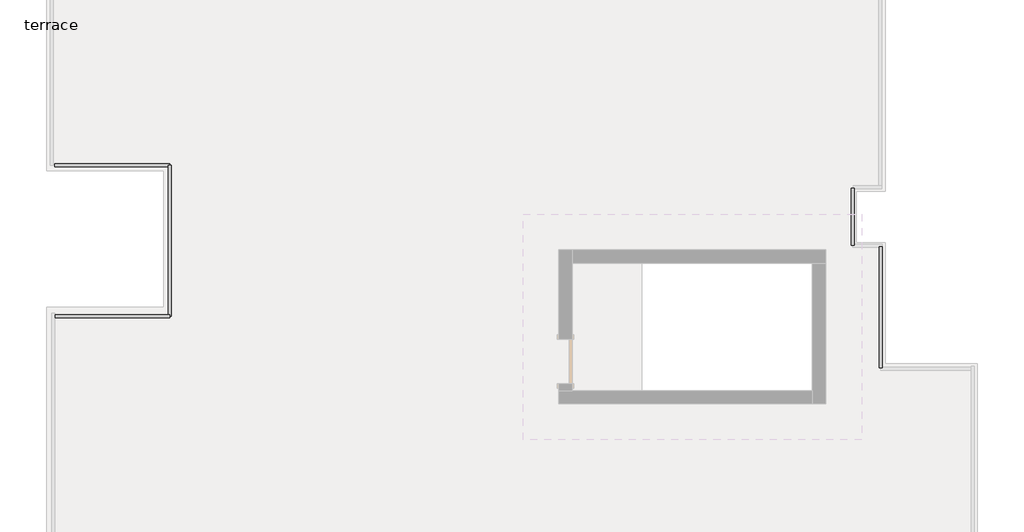
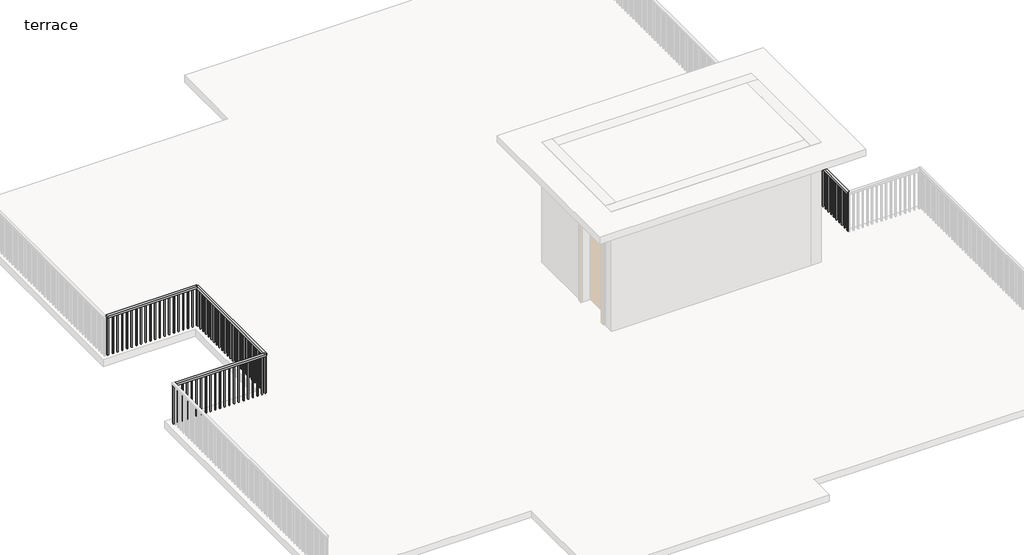
# One storey, part 4 of 7: 5 railings.
"""IFC4 building model written with IfcOpenShell, lengths in millimetres."""

from ifc_helpers import new_model, si_unit, frame, origin, place, context, project, spatial, polyline, outline, extrude, element, save

model = new_model("IFC4")

# Units and contexts
model_context = context("Model", 3, world=origin())
ifc_project = project(units=[si_unit("LENGTHUNIT", "METRE", prefix="MILLI")], contexts=[model_context])

# Site, building, storey
site = spatial("IfcSite", under=ifc_project)
building = spatial("IfcBuilding", under=site)
storey = spatial("IfcBuildingStorey", under=building, Name="terrace", Elevation=3810.0)

# Railings
placement = place(None, origin())
element("IfcRailing", 1, ObjectType="Handrail - Rectangular", at=placement, inside=storey, context=model_context, shape_type="SweptSolid", body=[
    extrude(outline(polyline([(-777.1890129, 5140.627622), (-726.3890129, 5140.627622), (-726.3890129, 4169.077622), (-777.1890129, 4169.077622), (-777.1890129, 5140.627622)])), frame((0.0, 0.0, 4673.6), z_axis=(0.0, 0.0, 1.0), x_axis=(1.0, 0.0, 0.0)), (0.0, 0.0, 1.0), 50.8),
    extrude(outline(polyline([(-761.3140129, 4235.752622), (-742.2640129, 4235.752622), (-742.2640129, 4216.702622), (-761.3140129, 4216.702622), (-761.3140129, 4235.752622)])), frame((0.0, 0.0, 3810.0), z_axis=(0.0, 0.0, 1.0), x_axis=(1.0, 0.0, 0.0)), (0.0, 0.0, 1.0), 863.6),
    extrude(outline(polyline([(-761.3140129, 4337.352622), (-742.2640129, 4337.352622), (-742.2640129, 4318.302622), (-761.3140129, 4318.302622), (-761.3140129, 4337.352622)])), frame((0.0, 0.0, 3810.0), z_axis=(0.0, 0.0, 1.0), x_axis=(1.0, 0.0, 0.0)), (0.0, 0.0, 1.0), 863.6),
    extrude(outline(polyline([(-761.3140129, 4438.952622), (-742.2640129, 4438.952622), (-742.2640129, 4419.902622), (-761.3140129, 4419.902622), (-761.3140129, 4438.952622)])), frame((0.0, 0.0, 3810.0), z_axis=(0.0, 0.0, 1.0), x_axis=(1.0, 0.0, 0.0)), (0.0, 0.0, 1.0), 863.6),
    extrude(outline(polyline([(-761.3140129, 4540.552622), (-742.2640129, 4540.552622), (-742.2640129, 4521.502622), (-761.3140129, 4521.502622), (-761.3140129, 4540.552622)])), frame((0.0, 0.0, 3810.0), z_axis=(0.0, 0.0, 1.0), x_axis=(1.0, 0.0, 0.0)), (0.0, 0.0, 1.0), 863.6),
    extrude(outline(polyline([(-761.3140129, 4642.152622), (-742.2640129, 4642.152622), (-742.2640129, 4623.102622), (-761.3140129, 4623.102622), (-761.3140129, 4642.152622)])), frame((0.0, 0.0, 3810.0), z_axis=(0.0, 0.0, 1.0), x_axis=(1.0, 0.0, 0.0)), (0.0, 0.0, 1.0), 863.6),
    extrude(outline(polyline([(-761.3140129, 4743.752622), (-742.2640129, 4743.752622), (-742.2640129, 4724.702622), (-761.3140129, 4724.702622), (-761.3140129, 4743.752622)])), frame((0.0, 0.0, 3810.0), z_axis=(0.0, 0.0, 1.0), x_axis=(1.0, 0.0, 0.0)), (0.0, 0.0, 1.0), 863.6),
    extrude(outline(polyline([(-761.3140129, 4845.352622), (-742.2640129, 4845.352622), (-742.2640129, 4826.302622), (-761.3140129, 4826.302622), (-761.3140129, 4845.352622)])), frame((0.0, 0.0, 3810.0), z_axis=(0.0, 0.0, 1.0), x_axis=(1.0, 0.0, 0.0)), (0.0, 0.0, 1.0), 863.6),
    extrude(outline(polyline([(-761.3140129, 4946.952622), (-742.2640129, 4946.952622), (-742.2640129, 4927.902622), (-761.3140129, 4927.902622), (-761.3140129, 4946.952622)])), frame((0.0, 0.0, 3810.0), z_axis=(0.0, 0.0, 1.0), x_axis=(1.0, 0.0, 0.0)), (0.0, 0.0, 1.0), 863.6),
    extrude(outline(polyline([(-761.3140129, 5048.552622), (-742.2640129, 5048.552622), (-742.2640129, 5029.502622), (-761.3140129, 5029.502622), (-761.3140129, 5048.552622)])), frame((0.0, 0.0, 3810.0), z_axis=(0.0, 0.0, 1.0), x_axis=(1.0, 0.0, 0.0)), (0.0, 0.0, 1.0), 863.6),
    extrude(outline(polyline([(-761.3140129, 4188.127622), (-742.2640129, 4188.127622), (-742.2640129, 4169.077622), (-761.3140129, 4169.077622), (-761.3140129, 4188.127622)])), frame((0.0, 0.0, 3810.0), z_axis=(0.0, 0.0, 1.0), x_axis=(1.0, 0.0, 0.0)), (0.0, 0.0, 1.0), 863.6),
    extrude(outline(polyline([(-761.3140129, 5140.627622), (-742.2640129, 5140.627622), (-742.2640129, 5121.577622), (-761.3140129, 5121.577622), (-761.3140129, 5140.627622)])), frame((0.0, 0.0, 3810.0), z_axis=(0.0, 0.0, 1.0), x_axis=(1.0, 0.0, 0.0)), (0.0, 0.0, 1.0), 863.6),
])
element("IfcRailing", 2, ObjectType="Handrail - Rectangular", at=placement, inside=storey, context=model_context, shape_type="SweptSolid", body=[
    extrude(outline(polyline([(-294.5890129, 4143.677622), (-243.7890129, 4143.677622), (-243.7890129, 2079.927622), (-294.5890129, 2079.927622), (-294.5890129, 4143.677622)])), frame((0.0, 0.0, 4673.6), z_axis=(0.0, 0.0, 1.0), x_axis=(1.0, 0.0, 0.0)), (0.0, 0.0, 1.0), 50.8),
    extrude(outline(polyline([(-278.7140129, 2121.202622), (-259.6640129, 2121.202622), (-259.6640129, 2102.152622), (-278.7140129, 2102.152622), (-278.7140129, 2121.202622)])), frame((0.0, 0.0, 3810.0), z_axis=(0.0, 0.0, 1.0), x_axis=(1.0, 0.0, 0.0)), (0.0, 0.0, 1.0), 863.6),
    extrude(outline(polyline([(-278.7140129, 2222.802622), (-259.6640129, 2222.802622), (-259.6640129, 2203.752622), (-278.7140129, 2203.752622), (-278.7140129, 2222.802622)])), frame((0.0, 0.0, 3810.0), z_axis=(0.0, 0.0, 1.0), x_axis=(1.0, 0.0, 0.0)), (0.0, 0.0, 1.0), 863.6),
    extrude(outline(polyline([(-278.7140129, 2324.402622), (-259.6640129, 2324.402622), (-259.6640129, 2305.352622), (-278.7140129, 2305.352622), (-278.7140129, 2324.402622)])), frame((0.0, 0.0, 3810.0), z_axis=(0.0, 0.0, 1.0), x_axis=(1.0, 0.0, 0.0)), (0.0, 0.0, 1.0), 863.6),
    extrude(outline(polyline([(-278.7140129, 2426.002622), (-259.6640129, 2426.002622), (-259.6640129, 2406.952622), (-278.7140129, 2406.952622), (-278.7140129, 2426.002622)])), frame((0.0, 0.0, 3810.0), z_axis=(0.0, 0.0, 1.0), x_axis=(1.0, 0.0, 0.0)), (0.0, 0.0, 1.0), 863.6),
    extrude(outline(polyline([(-278.7140129, 2527.602622), (-259.6640129, 2527.602622), (-259.6640129, 2508.552622), (-278.7140129, 2508.552622), (-278.7140129, 2527.602622)])), frame((0.0, 0.0, 3810.0), z_axis=(0.0, 0.0, 1.0), x_axis=(1.0, 0.0, 0.0)), (0.0, 0.0, 1.0), 863.6),
    extrude(outline(polyline([(-278.7140129, 2629.202622), (-259.6640129, 2629.202622), (-259.6640129, 2610.152622), (-278.7140129, 2610.152622), (-278.7140129, 2629.202622)])), frame((0.0, 0.0, 3810.0), z_axis=(0.0, 0.0, 1.0), x_axis=(1.0, 0.0, 0.0)), (0.0, 0.0, 1.0), 863.6),
    extrude(outline(polyline([(-278.7140129, 2730.802622), (-259.6640129, 2730.802622), (-259.6640129, 2711.752622), (-278.7140129, 2711.752622), (-278.7140129, 2730.802622)])), frame((0.0, 0.0, 3810.0), z_axis=(0.0, 0.0, 1.0), x_axis=(1.0, 0.0, 0.0)), (0.0, 0.0, 1.0), 863.6),
    extrude(outline(polyline([(-278.7140129, 2832.402622), (-259.6640129, 2832.402622), (-259.6640129, 2813.352622), (-278.7140129, 2813.352622), (-278.7140129, 2832.402622)])), frame((0.0, 0.0, 3810.0), z_axis=(0.0, 0.0, 1.0), x_axis=(1.0, 0.0, 0.0)), (0.0, 0.0, 1.0), 863.6),
    extrude(outline(polyline([(-278.7140129, 2934.002622), (-259.6640129, 2934.002622), (-259.6640129, 2914.952622), (-278.7140129, 2914.952622), (-278.7140129, 2934.002622)])), frame((0.0, 0.0, 3810.0), z_axis=(0.0, 0.0, 1.0), x_axis=(1.0, 0.0, 0.0)), (0.0, 0.0, 1.0), 863.6),
    extrude(outline(polyline([(-278.7140129, 3035.602622), (-259.6640129, 3035.602622), (-259.6640129, 3016.552622), (-278.7140129, 3016.552622), (-278.7140129, 3035.602622)])), frame((0.0, 0.0, 3810.0), z_axis=(0.0, 0.0, 1.0), x_axis=(1.0, 0.0, 0.0)), (0.0, 0.0, 1.0), 863.6),
    extrude(outline(polyline([(-278.7140129, 3137.202622), (-259.6640129, 3137.202622), (-259.6640129, 3118.152622), (-278.7140129, 3118.152622), (-278.7140129, 3137.202622)])), frame((0.0, 0.0, 3810.0), z_axis=(0.0, 0.0, 1.0), x_axis=(1.0, 0.0, 0.0)), (0.0, 0.0, 1.0), 863.6),
    extrude(outline(polyline([(-278.7140129, 3238.802622), (-259.6640129, 3238.802622), (-259.6640129, 3219.752622), (-278.7140129, 3219.752622), (-278.7140129, 3238.802622)])), frame((0.0, 0.0, 3810.0), z_axis=(0.0, 0.0, 1.0), x_axis=(1.0, 0.0, 0.0)), (0.0, 0.0, 1.0), 863.6),
    extrude(outline(polyline([(-278.7140129, 3340.402622), (-259.6640129, 3340.402622), (-259.6640129, 3321.352622), (-278.7140129, 3321.352622), (-278.7140129, 3340.402622)])), frame((0.0, 0.0, 3810.0), z_axis=(0.0, 0.0, 1.0), x_axis=(1.0, 0.0, 0.0)), (0.0, 0.0, 1.0), 863.6),
    extrude(outline(polyline([(-278.7140129, 3442.002622), (-259.6640129, 3442.002622), (-259.6640129, 3422.952622), (-278.7140129, 3422.952622), (-278.7140129, 3442.002622)])), frame((0.0, 0.0, 3810.0), z_axis=(0.0, 0.0, 1.0), x_axis=(1.0, 0.0, 0.0)), (0.0, 0.0, 1.0), 863.6),
    extrude(outline(polyline([(-278.7140129, 3543.602622), (-259.6640129, 3543.602622), (-259.6640129, 3524.552622), (-278.7140129, 3524.552622), (-278.7140129, 3543.602622)])), frame((0.0, 0.0, 3810.0), z_axis=(0.0, 0.0, 1.0), x_axis=(1.0, 0.0, 0.0)), (0.0, 0.0, 1.0), 863.6),
    extrude(outline(polyline([(-278.7140129, 3645.202622), (-259.6640129, 3645.202622), (-259.6640129, 3626.152622), (-278.7140129, 3626.152622), (-278.7140129, 3645.202622)])), frame((0.0, 0.0, 3810.0), z_axis=(0.0, 0.0, 1.0), x_axis=(1.0, 0.0, 0.0)), (0.0, 0.0, 1.0), 863.6),
    extrude(outline(polyline([(-278.7140129, 3746.802622), (-259.6640129, 3746.802622), (-259.6640129, 3727.752622), (-278.7140129, 3727.752622), (-278.7140129, 3746.802622)])), frame((0.0, 0.0, 3810.0), z_axis=(0.0, 0.0, 1.0), x_axis=(1.0, 0.0, 0.0)), (0.0, 0.0, 1.0), 863.6),
    extrude(outline(polyline([(-278.7140129, 3848.402622), (-259.6640129, 3848.402622), (-259.6640129, 3829.352622), (-278.7140129, 3829.352622), (-278.7140129, 3848.402622)])), frame((0.0, 0.0, 3810.0), z_axis=(0.0, 0.0, 1.0), x_axis=(1.0, 0.0, 0.0)), (0.0, 0.0, 1.0), 863.6),
    extrude(outline(polyline([(-278.7140129, 3950.002622), (-259.6640129, 3950.002622), (-259.6640129, 3930.952622), (-278.7140129, 3930.952622), (-278.7140129, 3950.002622)])), frame((0.0, 0.0, 3810.0), z_axis=(0.0, 0.0, 1.0), x_axis=(1.0, 0.0, 0.0)), (0.0, 0.0, 1.0), 863.6),
    extrude(outline(polyline([(-278.7140129, 4051.602622), (-259.6640129, 4051.602622), (-259.6640129, 4032.552622), (-278.7140129, 4032.552622), (-278.7140129, 4051.602622)])), frame((0.0, 0.0, 3810.0), z_axis=(0.0, 0.0, 1.0), x_axis=(1.0, 0.0, 0.0)), (0.0, 0.0, 1.0), 863.6),
    extrude(outline(polyline([(-278.7140129, 2098.977622), (-259.6640129, 2098.977622), (-259.6640129, 2079.927622), (-278.7140129, 2079.927622), (-278.7140129, 2098.977622)])), frame((0.0, 0.0, 3810.0), z_axis=(0.0, 0.0, 1.0), x_axis=(1.0, 0.0, 0.0)), (0.0, 0.0, 1.0), 863.6),
    extrude(outline(polyline([(-278.7140129, 4143.677622), (-259.6640129, 4143.677622), (-259.6640129, 4124.627622), (-278.7140129, 4124.627622), (-278.7140129, 4143.677622)])), frame((0.0, 0.0, 3810.0), z_axis=(0.0, 0.0, 1.0), x_axis=(1.0, 0.0, 0.0)), (0.0, 0.0, 1.0), 863.6),
])
element("IfcRailing", 3, ObjectType="Handrail - Rectangular", at=placement, inside=storey, context=model_context, shape_type="SweptSolid", body=[
    extrude(outline(polyline([(-14391.5890129, 2937.177622), (-14391.5890129, 2987.977622), (-12384.9890129, 2987.977622), (-12384.9890129, 2937.177622), (-14391.5890129, 2937.177622)])), frame((0.0, 0.0, 4673.6), z_axis=(0.0, 0.0, 1.0), x_axis=(1.0, 0.0, 0.0)), (0.0, 0.0, 1.0), 50.8),
    extrude(outline(polyline([(-12470.7140129, 2953.052622), (-12470.7140129, 2972.102622), (-12451.6640129, 2972.102622), (-12451.6640129, 2953.052622), (-12470.7140129, 2953.052622)])), frame((0.0, 0.0, 3810.0), z_axis=(0.0, 0.0, 1.0), x_axis=(1.0, 0.0, 0.0)), (0.0, 0.0, 1.0), 863.6),
    extrude(outline(polyline([(-12572.3140129, 2953.052622), (-12572.3140129, 2972.102622), (-12553.2640129, 2972.102622), (-12553.2640129, 2953.052622), (-12572.3140129, 2953.052622)])), frame((0.0, 0.0, 3810.0), z_axis=(0.0, 0.0, 1.0), x_axis=(1.0, 0.0, 0.0)), (0.0, 0.0, 1.0), 863.6),
    extrude(outline(polyline([(-12673.9140129, 2953.052622), (-12673.9140129, 2972.102622), (-12654.8640129, 2972.102622), (-12654.8640129, 2953.052622), (-12673.9140129, 2953.052622)])), frame((0.0, 0.0, 3810.0), z_axis=(0.0, 0.0, 1.0), x_axis=(1.0, 0.0, 0.0)), (0.0, 0.0, 1.0), 863.6),
    extrude(outline(polyline([(-12775.5140129, 2953.052622), (-12775.5140129, 2972.102622), (-12756.4640129, 2972.102622), (-12756.4640129, 2953.052622), (-12775.5140129, 2953.052622)])), frame((0.0, 0.0, 3810.0), z_axis=(0.0, 0.0, 1.0), x_axis=(1.0, 0.0, 0.0)), (0.0, 0.0, 1.0), 863.6),
    extrude(outline(polyline([(-12877.1140129, 2953.052622), (-12877.1140129, 2972.102622), (-12858.0640129, 2972.102622), (-12858.0640129, 2953.052622), (-12877.1140129, 2953.052622)])), frame((0.0, 0.0, 3810.0), z_axis=(0.0, 0.0, 1.0), x_axis=(1.0, 0.0, 0.0)), (0.0, 0.0, 1.0), 863.6),
    extrude(outline(polyline([(-12978.7140129, 2953.052622), (-12978.7140129, 2972.102622), (-12959.6640129, 2972.102622), (-12959.6640129, 2953.052622), (-12978.7140129, 2953.052622)])), frame((0.0, 0.0, 3810.0), z_axis=(0.0, 0.0, 1.0), x_axis=(1.0, 0.0, 0.0)), (0.0, 0.0, 1.0), 863.6),
    extrude(outline(polyline([(-13080.3140129, 2953.052622), (-13080.3140129, 2972.102622), (-13061.2640129, 2972.102622), (-13061.2640129, 2953.052622), (-13080.3140129, 2953.052622)])), frame((0.0, 0.0, 3810.0), z_axis=(0.0, 0.0, 1.0), x_axis=(1.0, 0.0, 0.0)), (0.0, 0.0, 1.0), 863.6),
    extrude(outline(polyline([(-13181.9140129, 2953.052622), (-13181.9140129, 2972.102622), (-13162.8640129, 2972.102622), (-13162.8640129, 2953.052622), (-13181.9140129, 2953.052622)])), frame((0.0, 0.0, 3810.0), z_axis=(0.0, 0.0, 1.0), x_axis=(1.0, 0.0, 0.0)), (0.0, 0.0, 1.0), 863.6),
    extrude(outline(polyline([(-13283.5140129, 2953.052622), (-13283.5140129, 2972.102622), (-13264.4640129, 2972.102622), (-13264.4640129, 2953.052622), (-13283.5140129, 2953.052622)])), frame((0.0, 0.0, 3810.0), z_axis=(0.0, 0.0, 1.0), x_axis=(1.0, 0.0, 0.0)), (0.0, 0.0, 1.0), 863.6),
    extrude(outline(polyline([(-13385.1140129, 2953.052622), (-13385.1140129, 2972.102622), (-13366.0640129, 2972.102622), (-13366.0640129, 2953.052622), (-13385.1140129, 2953.052622)])), frame((0.0, 0.0, 3810.0), z_axis=(0.0, 0.0, 1.0), x_axis=(1.0, 0.0, 0.0)), (0.0, 0.0, 1.0), 863.6),
    extrude(outline(polyline([(-13486.7140129, 2953.052622), (-13486.7140129, 2972.102622), (-13467.6640129, 2972.102622), (-13467.6640129, 2953.052622), (-13486.7140129, 2953.052622)])), frame((0.0, 0.0, 3810.0), z_axis=(0.0, 0.0, 1.0), x_axis=(1.0, 0.0, 0.0)), (0.0, 0.0, 1.0), 863.6),
    extrude(outline(polyline([(-13588.3140129, 2953.052622), (-13588.3140129, 2972.102622), (-13569.2640129, 2972.102622), (-13569.2640129, 2953.052622), (-13588.3140129, 2953.052622)])), frame((0.0, 0.0, 3810.0), z_axis=(0.0, 0.0, 1.0), x_axis=(1.0, 0.0, 0.0)), (0.0, 0.0, 1.0), 863.6),
    extrude(outline(polyline([(-13689.9140129, 2953.052622), (-13689.9140129, 2972.102622), (-13670.8640129, 2972.102622), (-13670.8640129, 2953.052622), (-13689.9140129, 2953.052622)])), frame((0.0, 0.0, 3810.0), z_axis=(0.0, 0.0, 1.0), x_axis=(1.0, 0.0, 0.0)), (0.0, 0.0, 1.0), 863.6),
    extrude(outline(polyline([(-13791.5140129, 2953.052622), (-13791.5140129, 2972.102622), (-13772.4640129, 2972.102622), (-13772.4640129, 2953.052622), (-13791.5140129, 2953.052622)])), frame((0.0, 0.0, 3810.0), z_axis=(0.0, 0.0, 1.0), x_axis=(1.0, 0.0, 0.0)), (0.0, 0.0, 1.0), 863.6),
    extrude(outline(polyline([(-13893.1140129, 2953.052622), (-13893.1140129, 2972.102622), (-13874.0640129, 2972.102622), (-13874.0640129, 2953.052622), (-13893.1140129, 2953.052622)])), frame((0.0, 0.0, 3810.0), z_axis=(0.0, 0.0, 1.0), x_axis=(1.0, 0.0, 0.0)), (0.0, 0.0, 1.0), 863.6),
    extrude(outline(polyline([(-13994.7140129, 2953.052622), (-13994.7140129, 2972.102622), (-13975.6640129, 2972.102622), (-13975.6640129, 2953.052622), (-13994.7140129, 2953.052622)])), frame((0.0, 0.0, 3810.0), z_axis=(0.0, 0.0, 1.0), x_axis=(1.0, 0.0, 0.0)), (0.0, 0.0, 1.0), 863.6),
    extrude(outline(polyline([(-14096.3140129, 2953.052622), (-14096.3140129, 2972.102622), (-14077.2640129, 2972.102622), (-14077.2640129, 2953.052622), (-14096.3140129, 2953.052622)])), frame((0.0, 0.0, 3810.0), z_axis=(0.0, 0.0, 1.0), x_axis=(1.0, 0.0, 0.0)), (0.0, 0.0, 1.0), 863.6),
    extrude(outline(polyline([(-14197.9140129, 2953.052622), (-14197.9140129, 2972.102622), (-14178.8640129, 2972.102622), (-14178.8640129, 2953.052622), (-14197.9140129, 2953.052622)])), frame((0.0, 0.0, 3810.0), z_axis=(0.0, 0.0, 1.0), x_axis=(1.0, 0.0, 0.0)), (0.0, 0.0, 1.0), 863.6),
    extrude(outline(polyline([(-14299.5140129, 2953.052622), (-14299.5140129, 2972.102622), (-14280.4640129, 2972.102622), (-14280.4640129, 2953.052622), (-14299.5140129, 2953.052622)])), frame((0.0, 0.0, 3810.0), z_axis=(0.0, 0.0, 1.0), x_axis=(1.0, 0.0, 0.0)), (0.0, 0.0, 1.0), 863.6),
    extrude(outline(polyline([(-12404.0390129, 2953.052622), (-12404.0390129, 2972.102622), (-12384.9890129, 2972.102622), (-12384.9890129, 2953.052622), (-12404.0390129, 2953.052622)])), frame((0.0, 0.0, 3810.0), z_axis=(0.0, 0.0, 1.0), x_axis=(1.0, 0.0, 0.0)), (0.0, 0.0, 1.0), 863.6),
    extrude(outline(polyline([(-14391.5890129, 2953.052622), (-14391.5890129, 2972.102622), (-14372.5390129, 2972.102622), (-14372.5390129, 2953.052622), (-14391.5890129, 2953.052622)])), frame((0.0, 0.0, 3810.0), z_axis=(0.0, 0.0, 1.0), x_axis=(1.0, 0.0, 0.0)), (0.0, 0.0, 1.0), 863.6),
])
element("IfcRailing", 4, ObjectType="Handrail - Rectangular", at=placement, inside=storey, context=model_context, shape_type="SweptSolid", body=[
    extrude(outline(polyline([(-12359.5890129, 2962.577622), (-12410.3890129, 2962.577622), (-12410.3890129, 5527.977622), (-12359.5890129, 5527.977622), (-12359.5890129, 2962.577622)])), frame((0.0, 0.0, 4673.6), z_axis=(0.0, 0.0, 1.0), x_axis=(1.0, 0.0, 0.0)), (0.0, 0.0, 1.0), 50.8),
    extrude(outline(polyline([(-12375.4640129, 5493.052622), (-12394.5140129, 5493.052622), (-12394.5140129, 5512.102622), (-12375.4640129, 5512.102622), (-12375.4640129, 5493.052622)])), frame((0.0, 0.0, 3810.0), z_axis=(0.0, 0.0, 1.0), x_axis=(1.0, 0.0, 0.0)), (0.0, 0.0, 1.0), 863.6),
    extrude(outline(polyline([(-12375.4640129, 5391.452622), (-12394.5140129, 5391.452622), (-12394.5140129, 5410.502622), (-12375.4640129, 5410.502622), (-12375.4640129, 5391.452622)])), frame((0.0, 0.0, 3810.0), z_axis=(0.0, 0.0, 1.0), x_axis=(1.0, 0.0, 0.0)), (0.0, 0.0, 1.0), 863.6),
    extrude(outline(polyline([(-12375.4640129, 5289.852622), (-12394.5140129, 5289.852622), (-12394.5140129, 5308.902622), (-12375.4640129, 5308.902622), (-12375.4640129, 5289.852622)])), frame((0.0, 0.0, 3810.0), z_axis=(0.0, 0.0, 1.0), x_axis=(1.0, 0.0, 0.0)), (0.0, 0.0, 1.0), 863.6),
    extrude(outline(polyline([(-12375.4640129, 5188.252622), (-12394.5140129, 5188.252622), (-12394.5140129, 5207.302622), (-12375.4640129, 5207.302622), (-12375.4640129, 5188.252622)])), frame((0.0, 0.0, 3810.0), z_axis=(0.0, 0.0, 1.0), x_axis=(1.0, 0.0, 0.0)), (0.0, 0.0, 1.0), 863.6),
    extrude(outline(polyline([(-12375.4640129, 5086.652622), (-12394.5140129, 5086.652622), (-12394.5140129, 5105.702622), (-12375.4640129, 5105.702622), (-12375.4640129, 5086.652622)])), frame((0.0, 0.0, 3810.0), z_axis=(0.0, 0.0, 1.0), x_axis=(1.0, 0.0, 0.0)), (0.0, 0.0, 1.0), 863.6),
    extrude(outline(polyline([(-12375.4640129, 4985.052622), (-12394.5140129, 4985.052622), (-12394.5140129, 5004.102622), (-12375.4640129, 5004.102622), (-12375.4640129, 4985.052622)])), frame((0.0, 0.0, 3810.0), z_axis=(0.0, 0.0, 1.0), x_axis=(1.0, 0.0, 0.0)), (0.0, 0.0, 1.0), 863.6),
    extrude(outline(polyline([(-12375.4640129, 4883.452622), (-12394.5140129, 4883.452622), (-12394.5140129, 4902.502622), (-12375.4640129, 4902.502622), (-12375.4640129, 4883.452622)])), frame((0.0, 0.0, 3810.0), z_axis=(0.0, 0.0, 1.0), x_axis=(1.0, 0.0, 0.0)), (0.0, 0.0, 1.0), 863.6),
    extrude(outline(polyline([(-12375.4640129, 4781.852622), (-12394.5140129, 4781.852622), (-12394.5140129, 4800.902622), (-12375.4640129, 4800.902622), (-12375.4640129, 4781.852622)])), frame((0.0, 0.0, 3810.0), z_axis=(0.0, 0.0, 1.0), x_axis=(1.0, 0.0, 0.0)), (0.0, 0.0, 1.0), 863.6),
    extrude(outline(polyline([(-12375.4640129, 4680.252622), (-12394.5140129, 4680.252622), (-12394.5140129, 4699.302622), (-12375.4640129, 4699.302622), (-12375.4640129, 4680.252622)])), frame((0.0, 0.0, 3810.0), z_axis=(0.0, 0.0, 1.0), x_axis=(1.0, 0.0, 0.0)), (0.0, 0.0, 1.0), 863.6),
    extrude(outline(polyline([(-12375.4640129, 4578.652622), (-12394.5140129, 4578.652622), (-12394.5140129, 4597.702622), (-12375.4640129, 4597.702622), (-12375.4640129, 4578.652622)])), frame((0.0, 0.0, 3810.0), z_axis=(0.0, 0.0, 1.0), x_axis=(1.0, 0.0, 0.0)), (0.0, 0.0, 1.0), 863.6),
    extrude(outline(polyline([(-12375.4640129, 4477.052622), (-12394.5140129, 4477.052622), (-12394.5140129, 4496.102622), (-12375.4640129, 4496.102622), (-12375.4640129, 4477.052622)])), frame((0.0, 0.0, 3810.0), z_axis=(0.0, 0.0, 1.0), x_axis=(1.0, 0.0, 0.0)), (0.0, 0.0, 1.0), 863.6),
    extrude(outline(polyline([(-12375.4640129, 4375.452622), (-12394.5140129, 4375.452622), (-12394.5140129, 4394.502622), (-12375.4640129, 4394.502622), (-12375.4640129, 4375.452622)])), frame((0.0, 0.0, 3810.0), z_axis=(0.0, 0.0, 1.0), x_axis=(1.0, 0.0, 0.0)), (0.0, 0.0, 1.0), 863.6),
    extrude(outline(polyline([(-12375.4640129, 4273.852622), (-12394.5140129, 4273.852622), (-12394.5140129, 4292.902622), (-12375.4640129, 4292.902622), (-12375.4640129, 4273.852622)])), frame((0.0, 0.0, 3810.0), z_axis=(0.0, 0.0, 1.0), x_axis=(1.0, 0.0, 0.0)), (0.0, 0.0, 1.0), 863.6),
    extrude(outline(polyline([(-12375.4640129, 4172.252622), (-12394.5140129, 4172.252622), (-12394.5140129, 4191.302622), (-12375.4640129, 4191.302622), (-12375.4640129, 4172.252622)])), frame((0.0, 0.0, 3810.0), z_axis=(0.0, 0.0, 1.0), x_axis=(1.0, 0.0, 0.0)), (0.0, 0.0, 1.0), 863.6),
    extrude(outline(polyline([(-12375.4640129, 4070.652622), (-12394.5140129, 4070.652622), (-12394.5140129, 4089.702622), (-12375.4640129, 4089.702622), (-12375.4640129, 4070.652622)])), frame((0.0, 0.0, 3810.0), z_axis=(0.0, 0.0, 1.0), x_axis=(1.0, 0.0, 0.0)), (0.0, 0.0, 1.0), 863.6),
    extrude(outline(polyline([(-12375.4640129, 3969.052622), (-12394.5140129, 3969.052622), (-12394.5140129, 3988.102622), (-12375.4640129, 3988.102622), (-12375.4640129, 3969.052622)])), frame((0.0, 0.0, 3810.0), z_axis=(0.0, 0.0, 1.0), x_axis=(1.0, 0.0, 0.0)), (0.0, 0.0, 1.0), 863.6),
    extrude(outline(polyline([(-12375.4640129, 3867.452622), (-12394.5140129, 3867.452622), (-12394.5140129, 3886.502622), (-12375.4640129, 3886.502622), (-12375.4640129, 3867.452622)])), frame((0.0, 0.0, 3810.0), z_axis=(0.0, 0.0, 1.0), x_axis=(1.0, 0.0, 0.0)), (0.0, 0.0, 1.0), 863.6),
    extrude(outline(polyline([(-12375.4640129, 3765.852622), (-12394.5140129, 3765.852622), (-12394.5140129, 3784.902622), (-12375.4640129, 3784.902622), (-12375.4640129, 3765.852622)])), frame((0.0, 0.0, 3810.0), z_axis=(0.0, 0.0, 1.0), x_axis=(1.0, 0.0, 0.0)), (0.0, 0.0, 1.0), 863.6),
    extrude(outline(polyline([(-12375.4640129, 3664.252622), (-12394.5140129, 3664.252622), (-12394.5140129, 3683.302622), (-12375.4640129, 3683.302622), (-12375.4640129, 3664.252622)])), frame((0.0, 0.0, 3810.0), z_axis=(0.0, 0.0, 1.0), x_axis=(1.0, 0.0, 0.0)), (0.0, 0.0, 1.0), 863.6),
    extrude(outline(polyline([(-12375.4640129, 3562.652622), (-12394.5140129, 3562.652622), (-12394.5140129, 3581.702622), (-12375.4640129, 3581.702622), (-12375.4640129, 3562.652622)])), frame((0.0, 0.0, 3810.0), z_axis=(0.0, 0.0, 1.0), x_axis=(1.0, 0.0, 0.0)), (0.0, 0.0, 1.0), 863.6),
    extrude(outline(polyline([(-12375.4640129, 3461.052622), (-12394.5140129, 3461.052622), (-12394.5140129, 3480.102622), (-12375.4640129, 3480.102622), (-12375.4640129, 3461.052622)])), frame((0.0, 0.0, 3810.0), z_axis=(0.0, 0.0, 1.0), x_axis=(1.0, 0.0, 0.0)), (0.0, 0.0, 1.0), 863.6),
    extrude(outline(polyline([(-12375.4640129, 3359.452622), (-12394.5140129, 3359.452622), (-12394.5140129, 3378.502622), (-12375.4640129, 3378.502622), (-12375.4640129, 3359.452622)])), frame((0.0, 0.0, 3810.0), z_axis=(0.0, 0.0, 1.0), x_axis=(1.0, 0.0, 0.0)), (0.0, 0.0, 1.0), 863.6),
    extrude(outline(polyline([(-12375.4640129, 3257.852622), (-12394.5140129, 3257.852622), (-12394.5140129, 3276.902622), (-12375.4640129, 3276.902622), (-12375.4640129, 3257.852622)])), frame((0.0, 0.0, 3810.0), z_axis=(0.0, 0.0, 1.0), x_axis=(1.0, 0.0, 0.0)), (0.0, 0.0, 1.0), 863.6),
    extrude(outline(polyline([(-12375.4640129, 3156.252622), (-12394.5140129, 3156.252622), (-12394.5140129, 3175.302622), (-12375.4640129, 3175.302622), (-12375.4640129, 3156.252622)])), frame((0.0, 0.0, 3810.0), z_axis=(0.0, 0.0, 1.0), x_axis=(1.0, 0.0, 0.0)), (0.0, 0.0, 1.0), 863.6),
    extrude(outline(polyline([(-12375.4640129, 3054.652622), (-12394.5140129, 3054.652622), (-12394.5140129, 3073.702622), (-12375.4640129, 3073.702622), (-12375.4640129, 3054.652622)])), frame((0.0, 0.0, 3810.0), z_axis=(0.0, 0.0, 1.0), x_axis=(1.0, 0.0, 0.0)), (0.0, 0.0, 1.0), 863.6),
    extrude(outline(polyline([(-12375.4640129, 5508.927622), (-12394.5140129, 5508.927622), (-12394.5140129, 5527.977622), (-12375.4640129, 5527.977622), (-12375.4640129, 5508.927622)])), frame((0.0, 0.0, 3810.0), z_axis=(0.0, 0.0, 1.0), x_axis=(1.0, 0.0, 0.0)), (0.0, 0.0, 1.0), 863.6),
    extrude(outline(polyline([(-12375.4640129, 2962.577622), (-12394.5140129, 2962.577622), (-12394.5140129, 2981.627622), (-12375.4640129, 2981.627622), (-12375.4640129, 2962.577622)])), frame((0.0, 0.0, 3810.0), z_axis=(0.0, 0.0, 1.0), x_axis=(1.0, 0.0, 0.0)), (0.0, 0.0, 1.0), 863.6),
])
element("IfcRailing", 5, ObjectType="Handrail - Rectangular", at=placement, inside=storey, context=model_context, shape_type="SweptSolid", body=[
    extrude(outline(polyline([(-12384.9890129, 5553.377622), (-12384.9890129, 5502.577622), (-14340.7890129, 5502.577622), (-14340.7890129, 5553.377622), (-12384.9890129, 5553.377622)])), frame((0.0, 0.0, 4673.6), z_axis=(0.0, 0.0, 1.0), x_axis=(1.0, 0.0, 0.0)), (0.0, 0.0, 1.0), 50.8),
    extrude(outline(polyline([(-14305.8640129, 5537.502622), (-14305.8640129, 5518.452622), (-14324.9140129, 5518.452622), (-14324.9140129, 5537.502622), (-14305.8640129, 5537.502622)])), frame((0.0, 0.0, 3810.0), z_axis=(0.0, 0.0, 1.0), x_axis=(1.0, 0.0, 0.0)), (0.0, 0.0, 1.0), 863.6),
    extrude(outline(polyline([(-14204.2640129, 5537.502622), (-14204.2640129, 5518.452622), (-14223.3140129, 5518.452622), (-14223.3140129, 5537.502622), (-14204.2640129, 5537.502622)])), frame((0.0, 0.0, 3810.0), z_axis=(0.0, 0.0, 1.0), x_axis=(1.0, 0.0, 0.0)), (0.0, 0.0, 1.0), 863.6),
    extrude(outline(polyline([(-14102.6640129, 5537.502622), (-14102.6640129, 5518.452622), (-14121.7140129, 5518.452622), (-14121.7140129, 5537.502622), (-14102.6640129, 5537.502622)])), frame((0.0, 0.0, 3810.0), z_axis=(0.0, 0.0, 1.0), x_axis=(1.0, 0.0, 0.0)), (0.0, 0.0, 1.0), 863.6),
    extrude(outline(polyline([(-14001.0640129, 5537.502622), (-14001.0640129, 5518.452622), (-14020.1140129, 5518.452622), (-14020.1140129, 5537.502622), (-14001.0640129, 5537.502622)])), frame((0.0, 0.0, 3810.0), z_axis=(0.0, 0.0, 1.0), x_axis=(1.0, 0.0, 0.0)), (0.0, 0.0, 1.0), 863.6),
    extrude(outline(polyline([(-13899.4640129, 5537.502622), (-13899.4640129, 5518.452622), (-13918.5140129, 5518.452622), (-13918.5140129, 5537.502622), (-13899.4640129, 5537.502622)])), frame((0.0, 0.0, 3810.0), z_axis=(0.0, 0.0, 1.0), x_axis=(1.0, 0.0, 0.0)), (0.0, 0.0, 1.0), 863.6),
    extrude(outline(polyline([(-13797.8640129, 5537.502622), (-13797.8640129, 5518.452622), (-13816.9140129, 5518.452622), (-13816.9140129, 5537.502622), (-13797.8640129, 5537.502622)])), frame((0.0, 0.0, 3810.0), z_axis=(0.0, 0.0, 1.0), x_axis=(1.0, 0.0, 0.0)), (0.0, 0.0, 1.0), 863.6),
    extrude(outline(polyline([(-13696.2640129, 5537.502622), (-13696.2640129, 5518.452622), (-13715.3140129, 5518.452622), (-13715.3140129, 5537.502622), (-13696.2640129, 5537.502622)])), frame((0.0, 0.0, 3810.0), z_axis=(0.0, 0.0, 1.0), x_axis=(1.0, 0.0, 0.0)), (0.0, 0.0, 1.0), 863.6),
    extrude(outline(polyline([(-13594.6640129, 5537.502622), (-13594.6640129, 5518.452622), (-13613.7140129, 5518.452622), (-13613.7140129, 5537.502622), (-13594.6640129, 5537.502622)])), frame((0.0, 0.0, 3810.0), z_axis=(0.0, 0.0, 1.0), x_axis=(1.0, 0.0, 0.0)), (0.0, 0.0, 1.0), 863.6),
    extrude(outline(polyline([(-13493.0640129, 5537.502622), (-13493.0640129, 5518.452622), (-13512.1140129, 5518.452622), (-13512.1140129, 5537.502622), (-13493.0640129, 5537.502622)])), frame((0.0, 0.0, 3810.0), z_axis=(0.0, 0.0, 1.0), x_axis=(1.0, 0.0, 0.0)), (0.0, 0.0, 1.0), 863.6),
    extrude(outline(polyline([(-13391.4640129, 5537.502622), (-13391.4640129, 5518.452622), (-13410.5140129, 5518.452622), (-13410.5140129, 5537.502622), (-13391.4640129, 5537.502622)])), frame((0.0, 0.0, 3810.0), z_axis=(0.0, 0.0, 1.0), x_axis=(1.0, 0.0, 0.0)), (0.0, 0.0, 1.0), 863.6),
    extrude(outline(polyline([(-13289.8640129, 5537.502622), (-13289.8640129, 5518.452622), (-13308.9140129, 5518.452622), (-13308.9140129, 5537.502622), (-13289.8640129, 5537.502622)])), frame((0.0, 0.0, 3810.0), z_axis=(0.0, 0.0, 1.0), x_axis=(1.0, 0.0, 0.0)), (0.0, 0.0, 1.0), 863.6),
    extrude(outline(polyline([(-13188.2640129, 5537.502622), (-13188.2640129, 5518.452622), (-13207.3140129, 5518.452622), (-13207.3140129, 5537.502622), (-13188.2640129, 5537.502622)])), frame((0.0, 0.0, 3810.0), z_axis=(0.0, 0.0, 1.0), x_axis=(1.0, 0.0, 0.0)), (0.0, 0.0, 1.0), 863.6),
    extrude(outline(polyline([(-13086.6640129, 5537.502622), (-13086.6640129, 5518.452622), (-13105.7140129, 5518.452622), (-13105.7140129, 5537.502622), (-13086.6640129, 5537.502622)])), frame((0.0, 0.0, 3810.0), z_axis=(0.0, 0.0, 1.0), x_axis=(1.0, 0.0, 0.0)), (0.0, 0.0, 1.0), 863.6),
    extrude(outline(polyline([(-12985.0640129, 5537.502622), (-12985.0640129, 5518.452622), (-13004.1140129, 5518.452622), (-13004.1140129, 5537.502622), (-12985.0640129, 5537.502622)])), frame((0.0, 0.0, 3810.0), z_axis=(0.0, 0.0, 1.0), x_axis=(1.0, 0.0, 0.0)), (0.0, 0.0, 1.0), 863.6),
    extrude(outline(polyline([(-12883.4640129, 5537.502622), (-12883.4640129, 5518.452622), (-12902.5140129, 5518.452622), (-12902.5140129, 5537.502622), (-12883.4640129, 5537.502622)])), frame((0.0, 0.0, 3810.0), z_axis=(0.0, 0.0, 1.0), x_axis=(1.0, 0.0, 0.0)), (0.0, 0.0, 1.0), 863.6),
    extrude(outline(polyline([(-12781.8640129, 5537.502622), (-12781.8640129, 5518.452622), (-12800.9140129, 5518.452622), (-12800.9140129, 5537.502622), (-12781.8640129, 5537.502622)])), frame((0.0, 0.0, 3810.0), z_axis=(0.0, 0.0, 1.0), x_axis=(1.0, 0.0, 0.0)), (0.0, 0.0, 1.0), 863.6),
    extrude(outline(polyline([(-12680.2640129, 5537.502622), (-12680.2640129, 5518.452622), (-12699.3140129, 5518.452622), (-12699.3140129, 5537.502622), (-12680.2640129, 5537.502622)])), frame((0.0, 0.0, 3810.0), z_axis=(0.0, 0.0, 1.0), x_axis=(1.0, 0.0, 0.0)), (0.0, 0.0, 1.0), 863.6),
    extrude(outline(polyline([(-12578.6640129, 5537.502622), (-12578.6640129, 5518.452622), (-12597.7140129, 5518.452622), (-12597.7140129, 5537.502622), (-12578.6640129, 5537.502622)])), frame((0.0, 0.0, 3810.0), z_axis=(0.0, 0.0, 1.0), x_axis=(1.0, 0.0, 0.0)), (0.0, 0.0, 1.0), 863.6),
    extrude(outline(polyline([(-12477.0640129, 5537.502622), (-12477.0640129, 5518.452622), (-12496.1140129, 5518.452622), (-12496.1140129, 5537.502622), (-12477.0640129, 5537.502622)])), frame((0.0, 0.0, 3810.0), z_axis=(0.0, 0.0, 1.0), x_axis=(1.0, 0.0, 0.0)), (0.0, 0.0, 1.0), 863.6),
    extrude(outline(polyline([(-14321.7390129, 5537.502622), (-14321.7390129, 5518.452622), (-14340.7890129, 5518.452622), (-14340.7890129, 5537.502622), (-14321.7390129, 5537.502622)])), frame((0.0, 0.0, 3810.0), z_axis=(0.0, 0.0, 1.0), x_axis=(1.0, 0.0, 0.0)), (0.0, 0.0, 1.0), 863.6),
    extrude(outline(polyline([(-12384.9890129, 5537.502622), (-12384.9890129, 5518.452622), (-12404.0390129, 5518.452622), (-12404.0390129, 5537.502622), (-12384.9890129, 5537.502622)])), frame((0.0, 0.0, 3810.0), z_axis=(0.0, 0.0, 1.0), x_axis=(1.0, 0.0, 0.0)), (0.0, 0.0, 1.0), 863.6),
])

save(model, "model.ifc")

# Revit data of these elements
# Type "Handrail - Rectangular"
#   Assembly Code = "C2010400"
#   built-in parameter 1008612 = 0.0416667 (stored number, unit not read)
#   built-in parameter 1008611 = 0.0416667 (stored number, unit not read)
#   built-in parameter 1008609 = 0.333333 (stored number, unit not read)
#   built-in parameter 1008604 = 0.166667 (stored number, unit not read)
#   built-in parameter 1008603 = 0.166667 (stored number, unit not read)
#   Railing Height = 3' - 0"
#   built-in parameter 1008630 = 2
#   built-in parameter 1008610 = 2
#   built-in parameter 1008618 = Baluster - Square : 3/4"
# Elements 1, 2, 3, 4, 5 (IfcRailing, "Handrail - Rectangular")
#   Phase Created = New Construction
